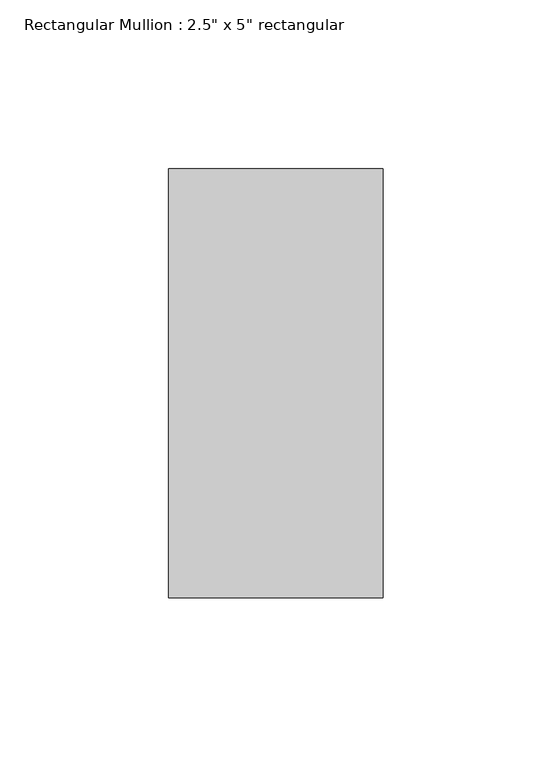
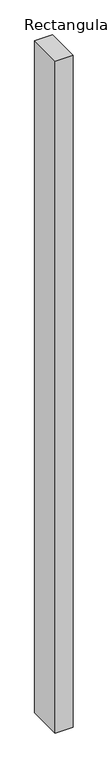
"""IFC4 building model written with IfcOpenShell, lengths in millimetres: member geometry."""

from ifc_helpers import new_model, si_unit, frame, origin, place, context, project, spatial, polyline, outline, extrude, source, transform, mapped, element, save


def member_be01e521(model_context):
    return source(origin(), model_context, "Body", "SweptSolid", [
        extrude(outline(polyline([(31.75, 63.5), (31.75, -63.5), (-31.75, -63.5), (-31.75, 63.5), (31.75, 63.5)])), frame((0.0, 0.0, -2538.6388159), z_axis=(0.0, 0.0, 1.0), x_axis=(1.0, 0.0, 0.0)), (0.0, 0.0, 1.0), 2538.6388159),
    ])


if __name__ == "__main__":
    model = new_model("IFC4")
    model_context = context("Model", 3, world=origin())
    ifc_project = project(units=[si_unit("LENGTHUNIT", "METRE", prefix="MILLI")], contexts=[model_context])
    site = spatial("IfcSite", under=ifc_project)
    building = spatial("IfcBuilding", under=site)
    placement = place(None, origin())
    member_shape = member_be01e521(model_context)
    element("IfcMember", 1, ObjectType="Rectangular Mullion : 2.5\" x 5\" rectangular", at=placement, inside=building, context=model_context, shape_type="MappedRepresentation", body=[
        mapped(member_shape, transform((0.0, 0.0, 0.0), x_axis=(1.0, 0.0, 0.0), y_axis=(0.0, 1.0, 0.0), z_axis=(0.0, 0.0, 1.0))),
    ])
    save(model, "model.ifc")

# Revit data of these elements
# Type "Rectangular Mullion : 2.5\" x 5\" rectangular"
#   built-in parameter 1007304 = 0.416667 (stored number, unit not read)
#   built-in parameter 1007301 = 0.104167 (stored number, unit not read)
#   built-in parameter 1007300 = 0.104167 (stored number, unit not read)
# Element 1 (IfcMember, "Rectangular Mullion : 2.5\" x 5\" rectangular")
#   Materials on its faces: "Aluminum"
# Materials
#   "Aluminum": class "Metal", colour RGB 247 247 247, transparency 0, Description = "Aluminum 6061", Cost = 0
